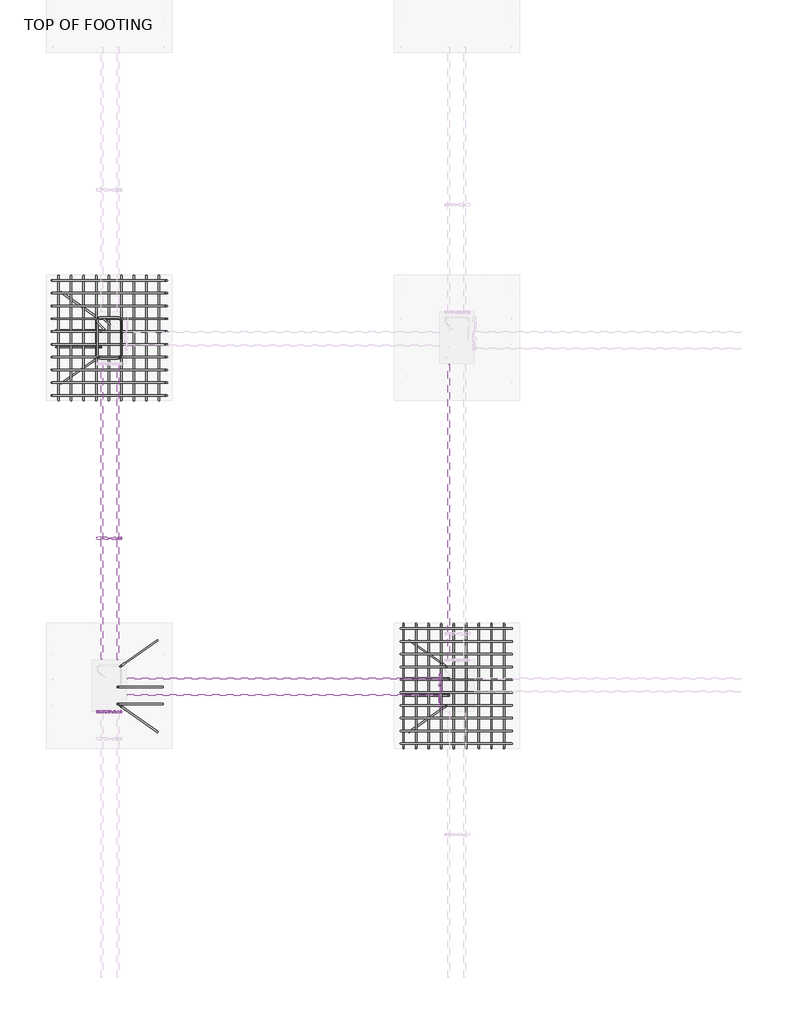
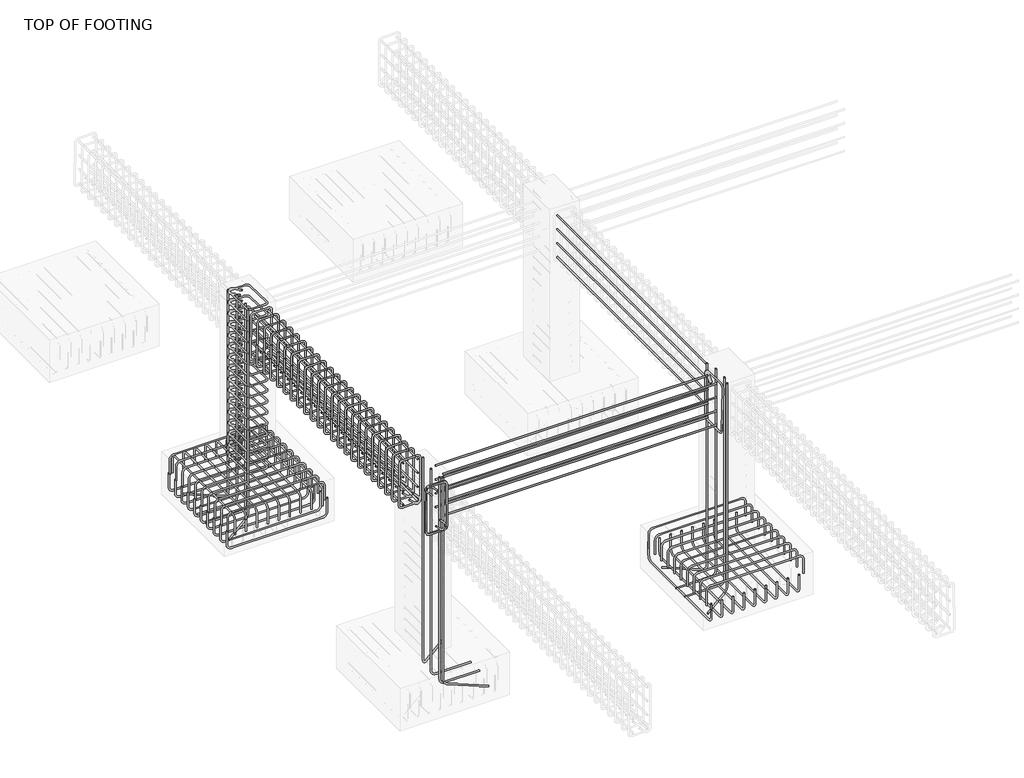
# One storey, part 6 of 18: 24 reinforcing bars.
"""IFC4 building model written with IfcOpenShell, lengths in millimetres."""

from ifc_helpers import new_model, si_unit, point, frame, origin, place, context, project, spatial, polyline, circle_curve, trimmed, segment, composite_curve, source, transform, mapped, element, save
from ifc_brep_helpers import swept_disk

model = new_model("IFC4")

# Units and contexts
model_context = context("Model", 3, world=origin())
ifc_project = project(units=[si_unit("LENGTHUNIT", "METRE", prefix="MILLI")], contexts=[model_context])

# Site, building, storey
site = spatial("IfcSite", under=ifc_project)
building = spatial("IfcBuilding", under=site)
storey = spatial("IfcBuildingStorey", under=building, Name="TOP OF FOOTING", Elevation=-1828.8)

# Reinforcing bars
placement = place(None, origin())
reinforcing_bar_shape = source(origin(), model_context, "Body", "SolidModel", [
    swept_disk(composite_curve([segment(polyline([(-11115.9859643, 12622.8477614, -40.0), (-11115.9859643, 12622.8477614, -2185.2530621)]), True, "CONTINUOUS"), segment(trimmed(circle_curve(frame((-11162.3359643, 12622.8477614, -2185.2530621), z_axis=(0.0, 1.0, 0.0), x_axis=(46.350000000000364, 0.0, 0.0)), 46.35), [point((-11115.9859643, 12622.8477614, -2185.2530621))], [point((-11162.3359643, 12622.8477614, -2231.6030621))], True, "CARTESIAN"), True, "CONTINUOUS"), segment(polyline([(-11162.3359643, 12622.8477614, -2231.6030621), (-11513.5126143, 12622.8477614, -2231.6030621)]), True, "CONTINUOUS")], self_intersect=False), 6.35),
])
element("IfcReinforcingBar", 1, at=placement, inside=storey, context=model_context, shape_type="MappedRepresentation", body=[
    mapped(reinforcing_bar_shape, transform((0.0, 0.0, 0.0), x_axis=(1.0, 0.0, 0.0), y_axis=(0.0, 1.0, 0.0), z_axis=(0.0, 0.0, 1.0))),
    mapped(reinforcing_bar_shape, transform((0.0, 148.3194112, 0.0), x_axis=(1.0, 0.0, 0.0), y_axis=(0.0, 1.0, 0.0), z_axis=(0.0, 0.0, 1.0))),
])
element("IfcReinforcingBar", 2, at=placement, inside=storey, context=model_context, shape_type="SolidModel", body=[
    swept_disk(composite_curve([segment(polyline([(-11140.9859643, 12878.3098681, -40.0), (-11140.9859643, 12878.3098681, -2185.2530621)]), True, "CONTINUOUS"), segment(trimmed(circle_curve(frame((-11178.9536616, 12904.895136, -2185.2530621), z_axis=(0.5735764363510552, 0.8191520442889856, 0.0), x_axis=(37.96769730000051, -26.585267899999963, 0.0)), 46.35), [point((-11140.9859643, 12878.3098681, -2185.2530621))], [point((-11178.9536616, 12904.895136, -2231.6030621))], True, "CARTESIAN"), True, "CONTINUOUS"), segment(polyline([(-11178.9536616, 12904.895136, -2231.6030621), (-11466.6207323, 13106.3217874, -2231.6030621)]), True, "CONTINUOUS")], self_intersect=False), 6.35),
])
reinforcing_bar_2_shape = source(origin(), model_context, "Body", "SolidModel", [
    swept_disk(composite_curve([segment(polyline([(-11036.6954038, 12818.3841028, -1782.45), (-11092.4389667, 12874.1276657, -1782.45)]), True, "CONTINUOUS"), segment(trimmed(circle_curve(frame((-11114.6067643, 12851.9598681, -1782.45), z_axis=(0.0, 0.0, 1.0), x_axis=(22.167797600000995, 22.167797599999176, 0.0)), 31.35), [point((-11092.4389667, 12874.1276657, -1782.45))], [point((-11145.9567643, 12851.9598681, -1782.45))], True, "CARTESIAN"), True, "CONTINUOUS"), segment(polyline([(-11145.9567643, 12851.9598681, -1782.45), (-11145.9567643, 12557.3598681, -1782.45)]), True, "CONTINUOUS"), segment(trimmed(circle_curve(frame((-11114.6067643, 12557.3598681, -1782.45), z_axis=(0.0, 0.0, 1.0), x_axis=(-31.349999999998545, 0.0, 0.0)), 31.35), [point((-11145.9567643, 12557.3598681, -1782.45))], [point((-11114.6067643, 12526.0098681, -1782.45))], True, "CARTESIAN"), True, "CONTINUOUS"), segment(polyline([(-11114.6067643, 12526.0098681, -1782.45), (-10970.0067643, 12526.0098681, -1782.45)]), True, "CONTINUOUS"), segment(trimmed(circle_curve(frame((-10970.0067643, 12557.3400831, -1783.5636125), z_axis=(0.0, 0.03552192833448158, 0.9993688971583016), x_axis=(0.0, -31.330214999999953, 1.1136125000000447)), 31.35), [point((-10970.0067643, 12526.0098681, -1782.45))], [point((-10938.6567643, 12557.3400831, -1783.5636125))], True, "CARTESIAN"), True, "CONTINUOUS"), segment(polyline([(-10938.6567643, 12557.3400831, -1783.5636125), (-10938.6567643, 12851.9796532, -1794.0363875)]), True, "CONTINUOUS"), segment(trimmed(circle_curve(frame((-10970.0067643, 12851.9796532, -1794.0363875), z_axis=(0.0, 0.03552192833448158, 0.9993688971583016), x_axis=(31.350000000000364, 0.0, 0.0)), 31.35), [point((-10938.6567643, 12851.9796532, -1794.0363875))], [point((-10970.0067643, 12883.3098681, -1795.15))], True, "CARTESIAN"), True, "CONTINUOUS"), segment(polyline([(-10970.0067643, 12883.3098681, -1795.15), (-11114.6067643, 12883.3098681, -1795.15)]), True, "CONTINUOUS"), segment(trimmed(circle_curve(frame((-11114.6067643, 12851.9598681, -1795.15), z_axis=(0.0, 0.0, 1.0), x_axis=(0.0, 31.349999999998545, 0.0)), 31.35), [point((-11114.6067643, 12883.3098681, -1795.15))], [point((-11136.7745619, 12829.7920705, -1795.15))], True, "CARTESIAN"), True, "CONTINUOUS"), segment(polyline([(-11136.7745619, 12829.7920705, -1795.15), (-11081.030999, 12774.0485076, -1795.15)]), True, "CONTINUOUS")], self_intersect=False), 6.35),
])
element("IfcReinforcingBar", 3, at=placement, inside=storey, context=model_context, shape_type="MappedRepresentation", body=[
    mapped(reinforcing_bar_2_shape, transform((0.0, 0.0, 0.0), x_axis=(1.0, 0.0, 0.0), y_axis=(0.0, 1.0, 0.0), z_axis=(0.0, 0.0, 1.0))),
    mapped(reinforcing_bar_2_shape, transform((0.0, 0.0, 116.0092918), x_axis=(1.0, 0.0, 0.0), y_axis=(0.0, 1.0, 0.0), z_axis=(0.0, 0.0, 1.0))),
    mapped(reinforcing_bar_2_shape, transform((0.0, 0.0, 232.0185836), x_axis=(1.0, 0.0, 0.0), y_axis=(0.0, 1.0, 0.0), z_axis=(0.0, 0.0, 1.0))),
    mapped(reinforcing_bar_2_shape, transform((0.0, 0.0, 348.0278755), x_axis=(1.0, 0.0, 0.0), y_axis=(0.0, 1.0, 0.0), z_axis=(0.0, 0.0, 1.0))),
    mapped(reinforcing_bar_2_shape, transform((0.0, 0.0, 464.0371673), x_axis=(1.0, 0.0, 0.0), y_axis=(0.0, 1.0, 0.0), z_axis=(0.0, 0.0, 1.0))),
    mapped(reinforcing_bar_2_shape, transform((0.0, 0.0, 580.0464591), x_axis=(1.0, 0.0, 0.0), y_axis=(0.0, 1.0, 0.0), z_axis=(0.0, 0.0, 1.0))),
    mapped(reinforcing_bar_2_shape, transform((0.0, 0.0, 696.0557509), x_axis=(1.0, 0.0, 0.0), y_axis=(0.0, 1.0, 0.0), z_axis=(0.0, 0.0, 1.0))),
    mapped(reinforcing_bar_2_shape, transform((0.0, 0.0, 812.0650428), x_axis=(1.0, 0.0, 0.0), y_axis=(0.0, 1.0, 0.0), z_axis=(0.0, 0.0, 1.0))),
    mapped(reinforcing_bar_2_shape, transform((0.0, 0.0, 928.0743346), x_axis=(1.0, 0.0, 0.0), y_axis=(0.0, 1.0, 0.0), z_axis=(0.0, 0.0, 1.0))),
    mapped(reinforcing_bar_2_shape, transform((0.0, 0.0, 1044.0836264), x_axis=(1.0, 0.0, 0.0), y_axis=(0.0, 1.0, 0.0), z_axis=(0.0, 0.0, 1.0))),
    mapped(reinforcing_bar_2_shape, transform((0.0, 0.0, 1160.0929182), x_axis=(1.0, 0.0, 0.0), y_axis=(0.0, 1.0, 0.0), z_axis=(0.0, 0.0, 1.0))),
    mapped(reinforcing_bar_2_shape, transform((0.0, 0.0, 1276.1022101), x_axis=(1.0, 0.0, 0.0), y_axis=(0.0, 1.0, 0.0), z_axis=(0.0, 0.0, 1.0))),
    mapped(reinforcing_bar_2_shape, transform((0.0, 0.0, 1392.1115019), x_axis=(1.0, 0.0, 0.0), y_axis=(0.0, 1.0, 0.0), z_axis=(0.0, 0.0, 1.0))),
    mapped(reinforcing_bar_2_shape, transform((0.0, 0.0, 1508.1207937), x_axis=(1.0, 0.0, 0.0), y_axis=(0.0, 1.0, 0.0), z_axis=(0.0, 0.0, 1.0))),
    mapped(reinforcing_bar_2_shape, transform((0.0, 0.0, 1624.1300855), x_axis=(1.0, 0.0, 0.0), y_axis=(0.0, 1.0, 0.0), z_axis=(0.0, 0.0, 1.0))),
    mapped(reinforcing_bar_2_shape, transform((0.0, 0.0, 1740.1393774), x_axis=(1.0, 0.0, 0.0), y_axis=(0.0, 1.0, 0.0), z_axis=(0.0, 0.0, 1.0))),
])
element("IfcReinforcingBar", 4, at=placement, inside=storey, context=model_context, shape_type="SolidModel", body=[
    swept_disk(composite_curve([segment(polyline([(-11140.9859643, 12531.0098681, -40.0), (-11140.9859643, 12531.0098681, -2185.2530621)]), True, "CONTINUOUS"), segment(trimmed(circle_curve(frame((-11178.9536616, 12504.4246003, -2185.2530621), z_axis=(-0.5735764363510106, 0.8191520442890168, 0.0), x_axis=(37.96769730000051, 26.5852677999992, 0.0)), 46.35), [point((-11140.9859643, 12531.0098681, -2185.2530621))], [point((-11178.9536616, 12504.4246003, -2231.6030621))], True, "CARTESIAN"), True, "CONTINUOUS"), segment(polyline([(-11178.9536616, 12504.4246003, -2231.6030621), (-11466.6207323, 12302.9979489, -2231.6030621)]), True, "CONTINUOUS")], self_intersect=False), 6.35),
])
element("IfcReinforcingBar", 5, at=placement, inside=storey, context=model_context, shape_type="SolidModel", body=[
    swept_disk(composite_curve([segment(polyline([(-10943.6275643, 9830.3098681, -40.0), (-10943.6275643, 9830.3098681, -2185.2530621)]), True, "CONTINUOUS"), segment(trimmed(circle_curve(frame((-10905.6598671, 9856.895136, -2185.2530621), z_axis=(0.5735764363510552, -0.8191520442889855, 0.0), x_axis=(-37.96769720000157, -26.585267899999963, 0.0)), 46.35), [point((-10943.6275643, 9830.3098681, -2185.2530621))], [point((-10905.6598671, 9856.895136, -2231.6030621))], True, "CARTESIAN"), True, "CONTINUOUS"), segment(polyline([(-10905.6598671, 9856.895136, -2231.6030621), (-10617.9927964, 10058.3217874, -2231.6030621)]), True, "CONTINUOUS")], self_intersect=False), 6.35),
])
element("IfcReinforcingBar", 6, at=placement, inside=storey, context=model_context, shape_type="SolidModel", body=[
    swept_disk(composite_curve([segment(polyline([(-10943.6275643, 9483.0098681, -40.0), (-10943.6275643, 9483.0098681, -2185.2530621)]), True, "CONTINUOUS"), segment(trimmed(circle_curve(frame((-10905.6598671, 9456.4246003, -2185.2530621), z_axis=(-0.5735764363510997, -0.8191520442889544, 0.0), x_axis=(-37.96769720000157, 26.5852677999992, 0.0)), 46.35), [point((-10943.6275643, 9483.0098681, -2185.2530621))], [point((-10905.6598671, 9456.4246003, -2231.6030621))], True, "CARTESIAN"), True, "CONTINUOUS"), segment(polyline([(-10905.6598671, 9456.4246003, -2231.6030621), (-10617.9927964, 9254.9979489, -2231.6030621)]), True, "CONTINUOUS")], self_intersect=False), 6.35),
])
reinforcing_bar_3_shape = source(origin(), model_context, "Body", "SolidModel", [
    swept_disk(composite_curve([segment(polyline([(-10968.6275643, 9499.8477614, -40.0), (-10968.6275643, 9499.8477614, -2185.2530621)]), True, "CONTINUOUS"), segment(trimmed(circle_curve(frame((-10922.2775643, 9499.8477614, -2185.2530621), z_axis=(0.0, -1.0, 0.0), x_axis=(-46.350000000000364, 0.0, 0.0)), 46.35), [point((-10968.6275643, 9499.8477614, -2185.2530621))], [point((-10922.2775643, 9499.8477614, -2231.6030621))], True, "CARTESIAN"), True, "CONTINUOUS"), segment(polyline([(-10922.2775643, 9499.8477614, -2231.6030621), (-10571.1009144, 9499.8477614, -2231.6030621)]), True, "CONTINUOUS")], self_intersect=False), 6.35),
])
element("IfcReinforcingBar", 7, at=placement, inside=storey, context=model_context, shape_type="MappedRepresentation", body=[
    mapped(reinforcing_bar_3_shape, transform((0.0, 0.0, 0.0), x_axis=(1.0, 0.0, 0.0), y_axis=(0.0, 1.0, 0.0), z_axis=(0.0, 0.0, 1.0))),
    mapped(reinforcing_bar_3_shape, transform((0.0, 148.3194112, 0.0), x_axis=(1.0, 0.0, 0.0), y_axis=(0.0, 1.0, 0.0), z_axis=(0.0, 0.0, 1.0))),
])
reinforcing_bar_4_shape = source(origin(), model_context, "Body", "SolidModel", [
    swept_disk(composite_curve([segment(polyline([(-8067.9859643, 9574.8477614, -40.0), (-8067.9859643, 9574.8477614, -2185.2530621)]), True, "CONTINUOUS"), segment(trimmed(circle_curve(frame((-8114.3359643, 9574.8477614, -2185.2530621), z_axis=(0.0, 1.0, 0.0), x_axis=(46.350000000000364, 0.0, 0.0)), 46.35), [point((-8067.9859643, 9574.8477614, -2185.2530621))], [point((-8114.3359643, 9574.8477614, -2231.6030621))], True, "CARTESIAN"), True, "CONTINUOUS"), segment(polyline([(-8114.3359643, 9574.8477614, -2231.6030621), (-8465.5126143, 9574.8477614, -2231.6030621)]), True, "CONTINUOUS")], self_intersect=False), 6.35),
])
element("IfcReinforcingBar", 8, at=placement, inside=storey, context=model_context, shape_type="MappedRepresentation", body=[
    mapped(reinforcing_bar_4_shape, transform((0.0, 0.0, 0.0), x_axis=(1.0, 0.0, 0.0), y_axis=(0.0, 1.0, 0.0), z_axis=(0.0, 0.0, 1.0))),
    mapped(reinforcing_bar_4_shape, transform((0.0, 148.3194112, 0.0), x_axis=(1.0, 0.0, 0.0), y_axis=(0.0, 1.0, 0.0), z_axis=(0.0, 0.0, 1.0))),
])
element("IfcReinforcingBar", 9, at=placement, inside=storey, context=model_context, shape_type="SolidModel", body=[
    swept_disk(composite_curve([segment(polyline([(-8092.9859643, 9830.3098681, -40.0), (-8092.9859643, 9830.3098681, -2185.2530621)]), True, "CONTINUOUS"), segment(trimmed(circle_curve(frame((-8130.9536616, 9856.895136, -2185.2530621), z_axis=(0.5735764363510552, 0.8191520442889855, 0.0), x_axis=(37.9676972999996, -26.585267899999963, 0.0)), 46.35), [point((-8092.9859643, 9830.3098681, -2185.2530621))], [point((-8130.9536616, 9856.895136, -2231.6030621))], True, "CARTESIAN"), True, "CONTINUOUS"), segment(polyline([(-8130.9536616, 9856.895136, -2231.6030621), (-8418.6207323, 10058.3217874, -2231.6030621)]), True, "CONTINUOUS")], self_intersect=False), 6.35),
])
element("IfcReinforcingBar", 10, at=placement, inside=storey, context=model_context, shape_type="SolidModel", body=[
    swept_disk(composite_curve([segment(polyline([(-8092.9859643, 9483.0098681, -40.0), (-8092.9859643, 9483.0098681, -2185.2530621)]), True, "CONTINUOUS"), segment(trimmed(circle_curve(frame((-8130.9536616, 9456.4246003, -2185.2530621), z_axis=(-0.5735764363510105, 0.8191520442890168, 0.0), x_axis=(37.9676972999996, 26.5852677999992, 0.0)), 46.35), [point((-8092.9859643, 9483.0098681, -2185.2530621))], [point((-8130.9536616, 9456.4246003, -2231.6030621))], True, "CARTESIAN"), True, "CONTINUOUS"), segment(polyline([(-8130.9536616, 9456.4246003, -2231.6030621), (-8418.6207323, 9254.9979489, -2231.6030621)]), True, "CONTINUOUS")], self_intersect=False), 6.35),
])
reinforcing_bar_5_shape = source(origin(), model_context, "Body", "SolidModel", [
    swept_disk(composite_curve([segment(polyline([(-8488.4399078, 10160.3098681, -2056.7800629), (-8488.4399078, 10160.3098681, -1909.4800629)]), True, "CONTINUOUS"), segment(trimmed(circle_curve(frame((-8442.0899078, 10160.3098681, -1909.4800629), z_axis=(0.0, 1.0, 0.0), x_axis=(-46.350000000000364, 0.0, 0.0)), 46.35), [point((-8488.4399078, 10160.3098681, -1909.4800629))], [point((-8442.0899078, 10160.3098681, -1863.1300629))], True, "CARTESIAN"), True, "CONTINUOUS"), segment(polyline([(-8442.0899078, 10160.3098681, -1863.1300629), (-7562.3320898, 10160.3098681, -1863.1300629)]), True, "CONTINUOUS"), segment(trimmed(circle_curve(frame((-7562.3320898, 10160.3098681, -1909.4800629), z_axis=(0.0, 1.0, 0.0), x_axis=(0.0, 0.0, 46.34999999999991)), 46.35), [point((-7562.3320898, 10160.3098681, -1863.1300629))], [point((-7515.9820898, 10160.3098681, -1909.4800629))], True, "CARTESIAN"), True, "CONTINUOUS"), segment(polyline([(-7515.9820898, 10160.3098681, -1909.4800629), (-7515.9820898, 10160.3098681, -2056.7800629)]), True, "CONTINUOUS")], self_intersect=False), 6.35),
])
element("IfcReinforcingBar", 11, at=placement, inside=storey, context=model_context, shape_type="MappedRepresentation", body=[
    mapped(reinforcing_bar_5_shape, transform((0.0, 0.0, 0.0), x_axis=(1.0, 0.0, 0.0), y_axis=(0.0, 1.0, 0.0), z_axis=(0.0, 0.0, 1.0))),
    mapped(reinforcing_bar_5_shape, transform((0.0, -111.9222222, 0.0), x_axis=(1.0, 0.0, 0.0), y_axis=(0.0, 1.0, 0.0), z_axis=(0.0, 0.0, 1.0))),
    mapped(reinforcing_bar_5_shape, transform((0.0, -223.8444444, 0.0), x_axis=(1.0, 0.0, 0.0), y_axis=(0.0, 1.0, 0.0), z_axis=(0.0, 0.0, 1.0))),
    mapped(reinforcing_bar_5_shape, transform((0.0, -335.7666667, 0.0), x_axis=(1.0, 0.0, 0.0), y_axis=(0.0, 1.0, 0.0), z_axis=(0.0, 0.0, 1.0))),
    mapped(reinforcing_bar_5_shape, transform((0.0, -447.6888889, 0.0), x_axis=(1.0, 0.0, 0.0), y_axis=(0.0, 1.0, 0.0), z_axis=(0.0, 0.0, 1.0))),
    mapped(reinforcing_bar_5_shape, transform((0.0, -559.6111111, 0.0), x_axis=(1.0, 0.0, 0.0), y_axis=(0.0, 1.0, 0.0), z_axis=(0.0, 0.0, 1.0))),
    mapped(reinforcing_bar_5_shape, transform((0.0, -671.5333333, 0.0), x_axis=(1.0, 0.0, 0.0), y_axis=(0.0, 1.0, 0.0), z_axis=(0.0, 0.0, 1.0))),
    mapped(reinforcing_bar_5_shape, transform((0.0, -783.4555556, 0.0), x_axis=(1.0, 0.0, 0.0), y_axis=(0.0, 1.0, 0.0), z_axis=(0.0, 0.0, 1.0))),
    mapped(reinforcing_bar_5_shape, transform((0.0, -895.3777778, 0.0), x_axis=(1.0, 0.0, 0.0), y_axis=(0.0, 1.0, 0.0), z_axis=(0.0, 0.0, 1.0))),
    mapped(reinforcing_bar_5_shape, transform((0.0, -1007.3, 0.0), x_axis=(1.0, 0.0, 0.0), y_axis=(0.0, 1.0, 0.0), z_axis=(0.0, 0.0, 1.0))),
])
reinforcing_bar_6_shape = source(origin(), model_context, "Body", "SolidModel", [
    swept_disk(composite_curve([segment(polyline([(-8465.5126143, 10200.3098681, -2025.2530621), (-8465.5126143, 10200.3098681, -2172.5530621)]), True, "CONTINUOUS"), segment(trimmed(circle_curve(frame((-8465.5126143, 10153.9598681, -2172.5530621), z_axis=(-1.0, 0.0, 0.0), x_axis=(0.0, 46.349999999998545, 0.0)), 46.35), [point((-8465.5126143, 10200.3098681, -2172.5530621))], [point((-8465.5126143, 10153.9598681, -2218.9030621))], True, "CARTESIAN"), True, "CONTINUOUS"), segment(polyline([(-8465.5126143, 10153.9598681, -2218.9030621), (-8465.5126143, 9159.3598681, -2218.9030621)]), True, "CONTINUOUS"), segment(trimmed(circle_curve(frame((-8465.5126143, 9159.3598681, -2172.5530621), z_axis=(-1.0, 0.0, 0.0), x_axis=(0.0, 0.0, -46.350000000000364)), 46.35), [point((-8465.5126143, 9159.3598681, -2218.9030621))], [point((-8465.5126143, 9113.0098681, -2172.5530621))], True, "CARTESIAN"), True, "CONTINUOUS"), segment(polyline([(-8465.5126143, 9113.0098681, -2172.5530621), (-8465.5126143, 9113.0098681, -2025.2530621)]), True, "CONTINUOUS")], self_intersect=False), 6.35),
])
element("IfcReinforcingBar", 12, at=placement, inside=storey, context=model_context, shape_type="MappedRepresentation", body=[
    mapped(reinforcing_bar_6_shape, transform((0.0, 0.0, 0.0), x_axis=(1.0, 0.0, 0.0), y_axis=(0.0, 1.0, 0.0), z_axis=(0.0, 0.0, 1.0))),
    mapped(reinforcing_bar_6_shape, transform((109.9890349, 0.0, 0.0), x_axis=(1.0, 0.0, 0.0), y_axis=(0.0, 1.0, 0.0), z_axis=(0.0, 0.0, 1.0))),
    mapped(reinforcing_bar_6_shape, transform((219.9780699, 0.0, 0.0), x_axis=(1.0, 0.0, 0.0), y_axis=(0.0, 1.0, 0.0), z_axis=(0.0, 0.0, 1.0))),
    mapped(reinforcing_bar_6_shape, transform((329.9671048, 0.0, 0.0), x_axis=(1.0, 0.0, 0.0), y_axis=(0.0, 1.0, 0.0), z_axis=(0.0, 0.0, 1.0))),
    mapped(reinforcing_bar_6_shape, transform((439.9561397, 0.0, 0.0), x_axis=(1.0, 0.0, 0.0), y_axis=(0.0, 1.0, 0.0), z_axis=(0.0, 0.0, 1.0))),
    mapped(reinforcing_bar_6_shape, transform((549.9451746, 0.0, 0.0), x_axis=(1.0, 0.0, 0.0), y_axis=(0.0, 1.0, 0.0), z_axis=(0.0, 0.0, 1.0))),
    mapped(reinforcing_bar_6_shape, transform((659.9342096, 0.0, 0.0), x_axis=(1.0, 0.0, 0.0), y_axis=(0.0, 1.0, 0.0), z_axis=(0.0, 0.0, 1.0))),
    mapped(reinforcing_bar_6_shape, transform((769.9232445, 0.0, 0.0), x_axis=(1.0, 0.0, 0.0), y_axis=(0.0, 1.0, 0.0), z_axis=(0.0, 0.0, 1.0))),
    mapped(reinforcing_bar_6_shape, transform((879.9122794, 0.0, 0.0), x_axis=(1.0, 0.0, 0.0), y_axis=(0.0, 1.0, 0.0), z_axis=(0.0, 0.0, 1.0))),
])
reinforcing_bar_7_shape = source(origin(), model_context, "Body", "SolidModel", [
    swept_disk(composite_curve([segment(polyline([(-10538.6567643, 13208.3098681, -2046.8654906), (-10538.6567643, 13208.3098681, -2194.1654906)]), True, "CONTINUOUS"), segment(trimmed(circle_curve(frame((-10585.0067643, 13208.3098681, -2194.1654906), z_axis=(0.0, 1.0, 0.0), x_axis=(46.350000000000364, 0.0, 0.0)), 46.35), [point((-10538.6567643, 13208.3098681, -2194.1654906))], [point((-10585.0067643, 13208.3098681, -2240.5154906))], True, "CARTESIAN"), True, "CONTINUOUS"), segment(polyline([(-10585.0067643, 13208.3098681, -2240.5154906), (-11499.6067643, 13208.3098681, -2240.5154906)]), True, "CONTINUOUS"), segment(trimmed(circle_curve(frame((-11499.6067643, 13208.3098681, -2194.1654906), z_axis=(0.0, 1.0, 0.0), x_axis=(0.0, 0.0, -46.34999999999991)), 46.35), [point((-11499.6067643, 13208.3098681, -2240.5154906))], [point((-11545.9567643, 13208.3098681, -2194.1654906))], True, "CARTESIAN"), True, "CONTINUOUS"), segment(polyline([(-11545.9567643, 13208.3098681, -2194.1654906), (-11545.9567643, 13208.3098681, -2046.8654906)]), True, "CONTINUOUS")], self_intersect=False), 6.35),
])
element("IfcReinforcingBar", 13, at=placement, inside=storey, context=model_context, shape_type="MappedRepresentation", body=[
    mapped(reinforcing_bar_7_shape, transform((0.0, 0.0, 0.0), x_axis=(1.0, 0.0, 0.0), y_axis=(0.0, 1.0, 0.0), z_axis=(0.0, 0.0, 1.0))),
    mapped(reinforcing_bar_7_shape, transform((0.0, -111.9222222, 0.0), x_axis=(1.0, 0.0, 0.0), y_axis=(0.0, 1.0, 0.0), z_axis=(0.0, 0.0, 1.0))),
    mapped(reinforcing_bar_7_shape, transform((0.0, -223.8444444, 0.0), x_axis=(1.0, 0.0, 0.0), y_axis=(0.0, 1.0, 0.0), z_axis=(0.0, 0.0, 1.0))),
    mapped(reinforcing_bar_7_shape, transform((0.0, -335.7666667, 0.0), x_axis=(1.0, 0.0, 0.0), y_axis=(0.0, 1.0, 0.0), z_axis=(0.0, 0.0, 1.0))),
    mapped(reinforcing_bar_7_shape, transform((0.0, -447.6888889, 0.0), x_axis=(1.0, 0.0, 0.0), y_axis=(0.0, 1.0, 0.0), z_axis=(0.0, 0.0, 1.0))),
    mapped(reinforcing_bar_7_shape, transform((0.0, -559.6111111, 0.0), x_axis=(1.0, 0.0, 0.0), y_axis=(0.0, 1.0, 0.0), z_axis=(0.0, 0.0, 1.0))),
    mapped(reinforcing_bar_7_shape, transform((0.0, -671.5333333, 0.0), x_axis=(1.0, 0.0, 0.0), y_axis=(0.0, 1.0, 0.0), z_axis=(0.0, 0.0, 1.0))),
    mapped(reinforcing_bar_7_shape, transform((0.0, -783.4555556, 0.0), x_axis=(1.0, 0.0, 0.0), y_axis=(0.0, 1.0, 0.0), z_axis=(0.0, 0.0, 1.0))),
    mapped(reinforcing_bar_7_shape, transform((0.0, -895.3777778, 0.0), x_axis=(1.0, 0.0, 0.0), y_axis=(0.0, 1.0, 0.0), z_axis=(0.0, 0.0, 1.0))),
    mapped(reinforcing_bar_7_shape, transform((0.0, -1007.3, 0.0), x_axis=(1.0, 0.0, 0.0), y_axis=(0.0, 1.0, 0.0), z_axis=(0.0, 0.0, 1.0))),
])
reinforcing_bar_8_shape = source(origin(), model_context, "Body", "SolidModel", [
    swept_disk(composite_curve([segment(polyline([(-11536.4399078, 13208.3098681, -2056.7800629), (-11536.4399078, 13208.3098681, -1909.4800629)]), True, "CONTINUOUS"), segment(trimmed(circle_curve(frame((-11490.0899078, 13208.3098681, -1909.4800629), z_axis=(0.0, 1.0, 0.0), x_axis=(-46.350000000000364, 0.0, 0.0)), 46.35), [point((-11536.4399078, 13208.3098681, -1909.4800629))], [point((-11490.0899078, 13208.3098681, -1863.1300629))], True, "CARTESIAN"), True, "CONTINUOUS"), segment(polyline([(-11490.0899078, 13208.3098681, -1863.1300629), (-10610.3320898, 13208.3098681, -1863.1300629)]), True, "CONTINUOUS"), segment(trimmed(circle_curve(frame((-10610.3320898, 13208.3098681, -1909.4800629), z_axis=(0.0, 1.0, 0.0), x_axis=(0.0, 0.0, 46.34999999999991)), 46.35), [point((-10610.3320898, 13208.3098681, -1863.1300629))], [point((-10563.9820898, 13208.3098681, -1909.4800629))], True, "CARTESIAN"), True, "CONTINUOUS"), segment(polyline([(-10563.9820898, 13208.3098681, -1909.4800629), (-10563.9820898, 13208.3098681, -2056.7800629)]), True, "CONTINUOUS")], self_intersect=False), 6.35),
])
element("IfcReinforcingBar", 14, at=placement, inside=storey, context=model_context, shape_type="MappedRepresentation", body=[
    mapped(reinforcing_bar_8_shape, transform((0.0, 0.0, 0.0), x_axis=(1.0, 0.0, 0.0), y_axis=(0.0, 1.0, 0.0), z_axis=(0.0, 0.0, 1.0))),
    mapped(reinforcing_bar_8_shape, transform((0.0, -111.9222222, 0.0), x_axis=(1.0, 0.0, 0.0), y_axis=(0.0, 1.0, 0.0), z_axis=(0.0, 0.0, 1.0))),
    mapped(reinforcing_bar_8_shape, transform((0.0, -223.8444444, 0.0), x_axis=(1.0, 0.0, 0.0), y_axis=(0.0, 1.0, 0.0), z_axis=(0.0, 0.0, 1.0))),
    mapped(reinforcing_bar_8_shape, transform((0.0, -335.7666667, 0.0), x_axis=(1.0, 0.0, 0.0), y_axis=(0.0, 1.0, 0.0), z_axis=(0.0, 0.0, 1.0))),
    mapped(reinforcing_bar_8_shape, transform((0.0, -447.6888889, 0.0), x_axis=(1.0, 0.0, 0.0), y_axis=(0.0, 1.0, 0.0), z_axis=(0.0, 0.0, 1.0))),
    mapped(reinforcing_bar_8_shape, transform((0.0, -559.6111111, 0.0), x_axis=(1.0, 0.0, 0.0), y_axis=(0.0, 1.0, 0.0), z_axis=(0.0, 0.0, 1.0))),
    mapped(reinforcing_bar_8_shape, transform((0.0, -671.5333333, 0.0), x_axis=(1.0, 0.0, 0.0), y_axis=(0.0, 1.0, 0.0), z_axis=(0.0, 0.0, 1.0))),
    mapped(reinforcing_bar_8_shape, transform((0.0, -783.4555556, 0.0), x_axis=(1.0, 0.0, 0.0), y_axis=(0.0, 1.0, 0.0), z_axis=(0.0, 0.0, 1.0))),
    mapped(reinforcing_bar_8_shape, transform((0.0, -895.3777778, 0.0), x_axis=(1.0, 0.0, 0.0), y_axis=(0.0, 1.0, 0.0), z_axis=(0.0, 0.0, 1.0))),
    mapped(reinforcing_bar_8_shape, transform((0.0, -1007.3, 0.0), x_axis=(1.0, 0.0, 0.0), y_axis=(0.0, 1.0, 0.0), z_axis=(0.0, 0.0, 1.0))),
])
reinforcing_bar_9_shape = source(origin(), model_context, "Body", "SolidModel", [
    swept_disk(composite_curve([segment(polyline([(-10607.1065918, 13248.3098681, -2080.1793981), (-10607.1065918, 13248.3098681, -1932.8793981)]), True, "CONTINUOUS"), segment(trimmed(circle_curve(frame((-10607.1065918, 13201.9598681, -1932.8793981), z_axis=(1.0, 0.0, 0.0), x_axis=(0.0, 46.349999999998545, 0.0)), 46.35), [point((-10607.1065918, 13248.3098681, -1932.8793981))], [point((-10607.1065918, 13201.9598681, -1886.5293981))], True, "CARTESIAN"), True, "CONTINUOUS"), segment(polyline([(-10607.1065918, 13201.9598681, -1886.5293981), (-10607.1065918, 12207.3598681, -1886.5293981)]), True, "CONTINUOUS"), segment(trimmed(circle_curve(frame((-10607.1065918, 12207.3598681, -1932.8793981), z_axis=(1.0, 0.0, 0.0), x_axis=(0.0, 0.0, 46.34999999999991)), 46.35), [point((-10607.1065918, 12207.3598681, -1886.5293981))], [point((-10607.1065918, 12161.0098681, -1932.8793981))], True, "CARTESIAN"), True, "CONTINUOUS"), segment(polyline([(-10607.1065918, 12161.0098681, -1932.8793981), (-10607.1065918, 12161.0098681, -2080.1793981)]), True, "CONTINUOUS")], self_intersect=False), 6.35),
])
element("IfcReinforcingBar", 15, at=placement, inside=storey, context=model_context, shape_type="MappedRepresentation", body=[
    mapped(reinforcing_bar_9_shape, transform((0.0, 0.0, 0.0), x_axis=(1.0, 0.0, 0.0), y_axis=(0.0, 1.0, 0.0), z_axis=(0.0, 0.0, 1.0))),
    mapped(reinforcing_bar_9_shape, transform((-109.9785589, 0.0, 0.0), x_axis=(1.0, 0.0, 0.0), y_axis=(0.0, 1.0, 0.0), z_axis=(0.0, 0.0, 1.0))),
    mapped(reinforcing_bar_9_shape, transform((-219.9571177, 0.0, 0.0), x_axis=(1.0, 0.0, 0.0), y_axis=(0.0, 1.0, 0.0), z_axis=(0.0, 0.0, 1.0))),
    mapped(reinforcing_bar_9_shape, transform((-329.9356766, 0.0, 0.0), x_axis=(1.0, 0.0, 0.0), y_axis=(0.0, 1.0, 0.0), z_axis=(0.0, 0.0, 1.0))),
    mapped(reinforcing_bar_9_shape, transform((-439.9142355, 0.0, 0.0), x_axis=(1.0, 0.0, 0.0), y_axis=(0.0, 1.0, 0.0), z_axis=(0.0, 0.0, 1.0))),
    mapped(reinforcing_bar_9_shape, transform((-549.8927943, 0.0, 0.0), x_axis=(1.0, 0.0, 0.0), y_axis=(0.0, 1.0, 0.0), z_axis=(0.0, 0.0, 1.0))),
    mapped(reinforcing_bar_9_shape, transform((-659.8713532, 0.0, 0.0), x_axis=(1.0, 0.0, 0.0), y_axis=(0.0, 1.0, 0.0), z_axis=(0.0, 0.0, 1.0))),
    mapped(reinforcing_bar_9_shape, transform((-769.8499121, 0.0, 0.0), x_axis=(1.0, 0.0, 0.0), y_axis=(0.0, 1.0, 0.0), z_axis=(0.0, 0.0, 1.0))),
    mapped(reinforcing_bar_9_shape, transform((-879.828471, 0.0, 0.0), x_axis=(1.0, 0.0, 0.0), y_axis=(0.0, 1.0, 0.0), z_axis=(0.0, 0.0, 1.0))),
])
reinforcing_bar_10_shape = source(origin(), model_context, "Body", "SolidModel", [
    swept_disk(composite_curve([segment(polyline([(-11047.9181249, 12473.3098681, -488.7242346), (-10992.1745619, 12473.3098681, -544.4677976)]), True, "CONTINUOUS"), segment(trimmed(circle_curve(frame((-10970.0067643, 12473.3098681, -522.3), z_axis=(0.0, -1.0, 0.0), x_axis=(-22.167797599999176, 0.0, -22.167797600000085)), 31.35), [point((-10992.1745619, 12473.3098681, -544.4677976))], [point((-10938.6567643, 12473.3098681, -522.3))], True, "CARTESIAN"), True, "CONTINUOUS"), segment(polyline([(-10938.6567643, 12473.3098681, -522.3), (-10938.6567643, 12473.3098681, -77.7)]), True, "CONTINUOUS"), segment(trimmed(circle_curve(frame((-10970.0067643, 12473.3098681, -77.7), z_axis=(0.0, -1.0, 0.0), x_axis=(31.350000000000364, 0.0, 0.0)), 31.35), [point((-10938.6567643, 12473.3098681, -77.7))], [point((-10970.0067643, 12473.3098681, -46.35))], True, "CARTESIAN"), True, "CONTINUOUS"), segment(polyline([(-10970.0067643, 12473.3098681, -46.35), (-11114.6067643, 12473.3098681, -46.35)]), True, "CONTINUOUS"), segment(trimmed(circle_curve(frame((-11114.6067643, 12474.0944538, -77.6901807), z_axis=(0.0, -0.9996867842138424, -0.025026655153786322), x_axis=(0.0, -0.7845857000011165, 31.340180699999998)), 31.35), [point((-11114.6067643, 12473.3098681, -46.35))], [point((-11145.9567643, 12474.0944538, -77.6901807))], True, "CARTESIAN"), True, "CONTINUOUS"), segment(polyline([(-11145.9567643, 12474.0944538, -77.6901807), (-11145.9567643, 12485.2252825, -522.3098193)]), True, "CONTINUOUS"), segment(trimmed(circle_curve(frame((-11114.6067643, 12485.2252825, -522.3098193), z_axis=(0.0, -0.9996867842138424, -0.025026655153786322), x_axis=(-31.349999999998545, 0.0, 0.0)), 31.35), [point((-11145.9567643, 12485.2252825, -522.3098193))], [point((-11114.6067643, 12486.0098681, -553.65))], True, "CARTESIAN"), True, "CONTINUOUS"), segment(polyline([(-11114.6067643, 12486.0098681, -553.65), (-10970.0067643, 12486.0098681, -553.65)]), True, "CONTINUOUS"), segment(trimmed(circle_curve(frame((-10970.0067643, 12486.0098681, -522.3), z_axis=(0.0, -1.0, 0.0), x_axis=(0.0, 0.0, -31.350000000000023)), 31.35), [point((-10970.0067643, 12486.0098681, -553.65))], [point((-10947.8389667, 12486.0098681, -500.1322024))], True, "CARTESIAN"), True, "CONTINUOUS"), segment(polyline([(-10947.8389667, 12486.0098681, -500.1322024), (-11003.5825297, 12486.0098681, -444.3886395)]), True, "CONTINUOUS")], self_intersect=False), 6.35),
])
element("IfcReinforcingBar", 16, at=placement, inside=storey, context=model_context, shape_type="MappedRepresentation", body=[
    mapped(reinforcing_bar_10_shape, transform((0.0, 0.0, 0.0), x_axis=(1.0, 0.0, 0.0), y_axis=(0.0, 1.0, 0.0), z_axis=(0.0, 0.0, 1.0))),
    mapped(reinforcing_bar_10_shape, transform((0.0, -117.5136364, 0.0), x_axis=(1.0, 0.0, 0.0), y_axis=(0.0, 1.0, 0.0), z_axis=(0.0, 0.0, 1.0))),
    mapped(reinforcing_bar_10_shape, transform((0.0, -235.0272727, 0.0), x_axis=(1.0, 0.0, 0.0), y_axis=(0.0, 1.0, 0.0), z_axis=(0.0, 0.0, 1.0))),
    mapped(reinforcing_bar_10_shape, transform((0.0, -352.5409091, 0.0), x_axis=(1.0, 0.0, 0.0), y_axis=(0.0, 1.0, 0.0), z_axis=(0.0, 0.0, 1.0))),
    mapped(reinforcing_bar_10_shape, transform((0.0, -470.0545455, 0.0), x_axis=(1.0, 0.0, 0.0), y_axis=(0.0, 1.0, 0.0), z_axis=(0.0, 0.0, 1.0))),
    mapped(reinforcing_bar_10_shape, transform((0.0, -587.5681818, 0.0), x_axis=(1.0, 0.0, 0.0), y_axis=(0.0, 1.0, 0.0), z_axis=(0.0, 0.0, 1.0))),
    mapped(reinforcing_bar_10_shape, transform((0.0, -705.0818182, 0.0), x_axis=(1.0, 0.0, 0.0), y_axis=(0.0, 1.0, 0.0), z_axis=(0.0, 0.0, 1.0))),
    mapped(reinforcing_bar_10_shape, transform((0.0, -822.5954545, 0.0), x_axis=(1.0, 0.0, 0.0), y_axis=(0.0, 1.0, 0.0), z_axis=(0.0, 0.0, 1.0))),
    mapped(reinforcing_bar_10_shape, transform((0.0, -940.1090909, 0.0), x_axis=(1.0, 0.0, 0.0), y_axis=(0.0, 1.0, 0.0), z_axis=(0.0, 0.0, 1.0))),
    mapped(reinforcing_bar_10_shape, transform((0.0, -1057.6227273, 0.0), x_axis=(1.0, 0.0, 0.0), y_axis=(0.0, 1.0, 0.0), z_axis=(0.0, 0.0, 1.0))),
    mapped(reinforcing_bar_10_shape, transform((0.0, -1175.1363636, 0.0), x_axis=(1.0, 0.0, 0.0), y_axis=(0.0, 1.0, 0.0), z_axis=(0.0, 0.0, 1.0))),
    mapped(reinforcing_bar_10_shape, transform((0.0, -1292.65, 0.0), x_axis=(1.0, 0.0, 0.0), y_axis=(0.0, 1.0, 0.0), z_axis=(0.0, 0.0, 1.0))),
    mapped(reinforcing_bar_10_shape, transform((0.0, -1410.1636364, 0.0), x_axis=(1.0, 0.0, 0.0), y_axis=(0.0, 1.0, 0.0), z_axis=(0.0, 0.0, 1.0))),
    mapped(reinforcing_bar_10_shape, transform((0.0, -1527.6772727, 0.0), x_axis=(1.0, 0.0, 0.0), y_axis=(0.0, 1.0, 0.0), z_axis=(0.0, 0.0, 1.0))),
    mapped(reinforcing_bar_10_shape, transform((0.0, -1645.1909091, 0.0), x_axis=(1.0, 0.0, 0.0), y_axis=(0.0, 1.0, 0.0), z_axis=(0.0, 0.0, 1.0))),
    mapped(reinforcing_bar_10_shape, transform((0.0, -1762.7045455, 0.0), x_axis=(1.0, 0.0, 0.0), y_axis=(0.0, 1.0, 0.0), z_axis=(0.0, 0.0, 1.0))),
    mapped(reinforcing_bar_10_shape, transform((0.0, -1880.2181818, 0.0), x_axis=(1.0, 0.0, 0.0), y_axis=(0.0, 1.0, 0.0), z_axis=(0.0, 0.0, 1.0))),
    mapped(reinforcing_bar_10_shape, transform((0.0, -1997.7318182, 0.0), x_axis=(1.0, 0.0, 0.0), y_axis=(0.0, 1.0, 0.0), z_axis=(0.0, 0.0, 1.0))),
    mapped(reinforcing_bar_10_shape, transform((0.0, -2115.2454545, 0.0), x_axis=(1.0, 0.0, 0.0), y_axis=(0.0, 1.0, 0.0), z_axis=(0.0, 0.0, 1.0))),
    mapped(reinforcing_bar_10_shape, transform((0.0, -2232.7590909, 0.0), x_axis=(1.0, 0.0, 0.0), y_axis=(0.0, 1.0, 0.0), z_axis=(0.0, 0.0, 1.0))),
    mapped(reinforcing_bar_10_shape, transform((0.0, -2350.2727273, 0.0), x_axis=(1.0, 0.0, 0.0), y_axis=(0.0, 1.0, 0.0), z_axis=(0.0, 0.0, 1.0))),
    mapped(reinforcing_bar_10_shape, transform((0.0, -2467.7863636, 0.0), x_axis=(1.0, 0.0, 0.0), y_axis=(0.0, 1.0, 0.0), z_axis=(0.0, 0.0, 1.0))),
    mapped(reinforcing_bar_10_shape, transform((0.0, -2585.3, 0.0), x_axis=(1.0, 0.0, 0.0), y_axis=(0.0, 1.0, 0.0), z_axis=(0.0, 0.0, 1.0))),
])
reinforcing_bar_11_shape = source(origin(), model_context, "Body", "SolidModel", [
    swept_disk(composite_curve([segment(polyline([(-10966.3740978, 12479.2648964, -524.1097861), (-10966.3740978, 9885.958437, -524.1097861)]), True, "CONTINUOUS")], self_intersect=False), 6.35),
])
element("IfcReinforcingBar", 17, at=placement, inside=storey, context=model_context, shape_type="MappedRepresentation", body=[
    mapped(reinforcing_bar_11_shape, transform((0.0, 0.0, 0.0), x_axis=(1.0, 0.0, 0.0), y_axis=(0.0, 1.0, 0.0), z_axis=(0.0, 0.0, 1.0))),
    mapped(reinforcing_bar_11_shape, transform((0.0, 0.0, 147.1005596), x_axis=(1.0, 0.0, 0.0), y_axis=(0.0, 1.0, 0.0), z_axis=(0.0, 0.0, 1.0))),
    mapped(reinforcing_bar_11_shape, transform((0.0, 0.0, 294.2011193), x_axis=(1.0, 0.0, 0.0), y_axis=(0.0, 1.0, 0.0), z_axis=(0.0, 0.0, 1.0))),
    mapped(reinforcing_bar_11_shape, transform((0.0, 0.0, 441.3016789), x_axis=(1.0, 0.0, 0.0), y_axis=(0.0, 1.0, 0.0), z_axis=(0.0, 0.0, 1.0))),
])
reinforcing_bar_12_shape = source(origin(), model_context, "Body", "SolidModel", [
    swept_disk(composite_curve([segment(polyline([(-11108.2394308, 12474.6455035, -524.1097861), (-11108.2394308, 9891.9745179, -524.1097861)]), True, "CONTINUOUS")], self_intersect=False), 6.35),
])
element("IfcReinforcingBar", 18, at=placement, inside=storey, context=model_context, shape_type="MappedRepresentation", body=[
    mapped(reinforcing_bar_12_shape, transform((0.0, 0.0, 0.0), x_axis=(1.0, 0.0, 0.0), y_axis=(0.0, 1.0, 0.0), z_axis=(0.0, 0.0, 1.0))),
    mapped(reinforcing_bar_12_shape, transform((0.0, 0.0, 147.1005596), x_axis=(1.0, 0.0, 0.0), y_axis=(0.0, 1.0, 0.0), z_axis=(0.0, 0.0, 1.0))),
    mapped(reinforcing_bar_12_shape, transform((0.0, 0.0, 294.2011193), x_axis=(1.0, 0.0, 0.0), y_axis=(0.0, 1.0, 0.0), z_axis=(0.0, 0.0, 1.0))),
    mapped(reinforcing_bar_12_shape, transform((0.0, 0.0, 441.3016789), x_axis=(1.0, 0.0, 0.0), y_axis=(0.0, 1.0, 0.0), z_axis=(0.0, 0.0, 1.0))),
])
element("IfcReinforcingBar", 19, at=placement, inside=storey, context=model_context, shape_type="SolidModel", body=[
    swept_disk(composite_curve([segment(polyline([(-11036.6954038, 9425.3098681, -111.2757654), (-11092.4389667, 9425.3098681, -55.5322024)]), True, "CONTINUOUS"), segment(trimmed(circle_curve(frame((-11114.6067643, 9425.3098681, -77.7), z_axis=(0.0, -1.0, 0.0), x_axis=(22.167797600000995, 0.0, 22.1677976)), 31.35), [point((-11092.4389667, 9425.3098681, -55.5322024))], [point((-11145.9567643, 9425.3098681, -77.7))], True, "CARTESIAN"), True, "CONTINUOUS"), segment(polyline([(-11145.9567643, 9425.3098681, -77.7), (-11145.9567643, 9425.3098681, -522.3)]), True, "CONTINUOUS"), segment(trimmed(circle_curve(frame((-11114.6067643, 9425.3098681, -522.3), z_axis=(0.0, -1.0, 0.0), x_axis=(-31.349999999998545, 0.0, 0.0)), 31.35), [point((-11145.9567643, 9425.3098681, -522.3))], [point((-11114.6067643, 9425.3098681, -553.65))], True, "CARTESIAN"), True, "CONTINUOUS"), segment(polyline([(-11114.6067643, 9425.3098681, -553.65), (-10970.0067643, 9425.3098681, -553.65)]), True, "CONTINUOUS"), segment(trimmed(circle_curve(frame((-10970.0067643, 9426.0944538, -522.3098193), z_axis=(0.0, -0.9996867842138424, 0.025026655153786322), x_axis=(0.0, -0.7845857000011165, -31.34018070000002)), 31.35), [point((-10970.0067643, 9425.3098681, -553.65))], [point((-10938.6567643, 9426.0944538, -522.3098193))], True, "CARTESIAN"), True, "CONTINUOUS"), segment(polyline([(-10938.6567643, 9426.0944538, -522.3098193), (-10938.6567643, 9437.2252825, -77.6901807)]), True, "CONTINUOUS"), segment(trimmed(circle_curve(frame((-10970.0067643, 9437.2252825, -77.6901807), z_axis=(0.0, -0.9996867842138424, 0.025026655153786322), x_axis=(31.350000000000364, 0.0, 0.0)), 31.35), [point((-10938.6567643, 9437.2252825, -77.6901807))], [point((-10970.0067643, 9438.0098681, -46.35))], True, "CARTESIAN"), True, "CONTINUOUS"), segment(polyline([(-10970.0067643, 9438.0098681, -46.35), (-11114.6067643, 9438.0098681, -46.35)]), True, "CONTINUOUS"), segment(trimmed(circle_curve(frame((-11114.6067643, 9438.0098681, -77.7), z_axis=(0.0, -1.0, 0.0), x_axis=(0.0, 0.0, 31.35)), 31.35), [point((-11114.6067643, 9438.0098681, -46.35))], [point((-11136.7745619, 9438.0098681, -99.8677976))], True, "CARTESIAN"), True, "CONTINUOUS"), segment(polyline([(-11136.7745619, 9438.0098681, -99.8677976), (-11081.030999, 9438.0098681, -155.6113605)]), True, "CONTINUOUS")], self_intersect=False), 6.35),
])
element("IfcReinforcingBar", 20, at=placement, inside=storey, context=model_context, shape_type="SolidModel", body=[
    swept_disk(composite_curve([segment(polyline([(-11047.9181249, 9425.3098681, -488.7242346), (-10992.1745619, 9425.3098681, -544.4677976)]), True, "CONTINUOUS"), segment(trimmed(circle_curve(frame((-10970.0067643, 9425.3098681, -522.3), z_axis=(0.0, -1.0, 0.0), x_axis=(-22.167797599999176, 0.0, -22.167797600000085)), 31.35), [point((-10992.1745619, 9425.3098681, -544.4677976))], [point((-10938.6567643, 9425.3098681, -522.3))], True, "CARTESIAN"), True, "CONTINUOUS"), segment(polyline([(-10938.6567643, 9425.3098681, -522.3), (-10938.6567643, 9425.3098681, -77.7)]), True, "CONTINUOUS"), segment(trimmed(circle_curve(frame((-10970.0067643, 9425.3098681, -77.7), z_axis=(0.0, -1.0, 0.0), x_axis=(31.350000000000364, 0.0, 0.0)), 31.35), [point((-10938.6567643, 9425.3098681, -77.7))], [point((-10970.0067643, 9425.3098681, -46.35))], True, "CARTESIAN"), True, "CONTINUOUS"), segment(polyline([(-10970.0067643, 9425.3098681, -46.35), (-11114.6067643, 9425.3098681, -46.35)]), True, "CONTINUOUS"), segment(trimmed(circle_curve(frame((-11114.6067643, 9426.0944538, -77.6901807), z_axis=(0.0, -0.9996867842138424, -0.025026655153786322), x_axis=(0.0, -0.7845857000011165, 31.340180699999998)), 31.35), [point((-11114.6067643, 9425.3098681, -46.35))], [point((-11145.9567643, 9426.0944538, -77.6901807))], True, "CARTESIAN"), True, "CONTINUOUS"), segment(polyline([(-11145.9567643, 9426.0944538, -77.6901807), (-11145.9567643, 9437.2252825, -522.3098193)]), True, "CONTINUOUS"), segment(trimmed(circle_curve(frame((-11114.6067643, 9437.2252825, -522.3098193), z_axis=(0.0, -0.9996867842138424, -0.025026655153786322), x_axis=(-31.349999999998545, 0.0, 0.0)), 31.35), [point((-11145.9567643, 9437.2252825, -522.3098193))], [point((-11114.6067643, 9438.0098681, -553.65))], True, "CARTESIAN"), True, "CONTINUOUS"), segment(polyline([(-11114.6067643, 9438.0098681, -553.65), (-10970.0067643, 9438.0098681, -553.65)]), True, "CONTINUOUS"), segment(trimmed(circle_curve(frame((-10970.0067643, 9438.0098681, -522.3), z_axis=(0.0, -1.0, 0.0), x_axis=(0.0, 0.0, -31.350000000000023)), 31.35), [point((-10970.0067643, 9438.0098681, -553.65))], [point((-10947.8389667, 9438.0098681, -500.1322024))], True, "CARTESIAN"), True, "CONTINUOUS"), segment(polyline([(-10947.8389667, 9438.0098681, -500.1322024), (-11003.5825297, 9438.0098681, -444.3886395)]), True, "CONTINUOUS")], self_intersect=False), 6.35),
])
reinforcing_bar_13_shape = source(origin(), model_context, "Body", "SolidModel", [
    swept_disk(composite_curve([segment(polyline([(-8070.2394308, 9882.0548399, -524.1097861), (-8070.2394308, 12475.3612993, -524.1097861)]), True, "CONTINUOUS")], self_intersect=False), 6.35),
])
element("IfcReinforcingBar", 21, at=placement, inside=storey, context=model_context, shape_type="MappedRepresentation", body=[
    mapped(reinforcing_bar_13_shape, transform((0.0, 0.0, 0.0), x_axis=(1.0, 0.0, 0.0), y_axis=(0.0, 1.0, 0.0), z_axis=(0.0, 0.0, 1.0))),
    mapped(reinforcing_bar_13_shape, transform((0.0, 0.0, 147.1005596), x_axis=(1.0, 0.0, 0.0), y_axis=(0.0, 1.0, 0.0), z_axis=(0.0, 0.0, 1.0))),
    mapped(reinforcing_bar_13_shape, transform((0.0, 0.0, 294.2011193), x_axis=(1.0, 0.0, 0.0), y_axis=(0.0, 1.0, 0.0), z_axis=(0.0, 0.0, 1.0))),
    mapped(reinforcing_bar_13_shape, transform((0.0, 0.0, 441.3016789), x_axis=(1.0, 0.0, 0.0), y_axis=(0.0, 1.0, 0.0), z_axis=(0.0, 0.0, 1.0))),
])
element("IfcReinforcingBar", 22, at=placement, inside=storey, context=model_context, shape_type="SolidModel", body=[
    swept_disk(composite_curve([segment(polyline([(-8150.6567643, 9651.0485076, -111.2757654), (-8150.6567643, 9706.7920705, -55.5322024)]), True, "CONTINUOUS"), segment(trimmed(circle_curve(frame((-8150.6567643, 9728.9598681, -77.7), z_axis=(-1.0, 0.0, 0.0), x_axis=(0.0, -22.167797600000995, 22.1677976)), 31.35), [point((-8150.6567643, 9706.7920705, -55.5322024))], [point((-8150.6567643, 9760.3098681, -77.7))], True, "CARTESIAN"), True, "CONTINUOUS"), segment(polyline([(-8150.6567643, 9760.3098681, -77.7), (-8150.6567643, 9760.3098681, -522.3)]), True, "CONTINUOUS"), segment(trimmed(circle_curve(frame((-8150.6567643, 9728.9598681, -522.3), z_axis=(-1.0, 0.0, 0.0), x_axis=(0.0, 31.349999999998545, 0.0)), 31.35), [point((-8150.6567643, 9760.3098681, -522.3))], [point((-8150.6567643, 9728.9598681, -553.65))], True, "CARTESIAN"), True, "CONTINUOUS"), segment(polyline([(-8150.6567643, 9728.9598681, -553.65), (-8150.6567643, 9509.3598681, -553.65)]), True, "CONTINUOUS"), segment(trimmed(circle_curve(frame((-8149.8721787, 9509.3598681, -522.3098193), z_axis=(-0.9996867842138424, 0.0, 0.025026655153786322), x_axis=(-0.7845855999994455, 0.0, -31.34018070000002)), 31.35), [point((-8150.6567643, 9509.3598681, -553.65))], [point((-8149.8721787, 9478.0098681, -522.3098193))], True, "CARTESIAN"), True, "CONTINUOUS"), segment(polyline([(-8149.8721787, 9478.0098681, -522.3098193), (-8138.74135, 9478.0098681, -77.6901807)]), True, "CONTINUOUS"), segment(trimmed(circle_curve(frame((-8138.74135, 9509.3598681, -77.6901807), z_axis=(-0.9996867842138424, 0.0, 0.025026655153786322), x_axis=(0.0, -31.350000000000364, 0.0)), 31.35), [point((-8138.74135, 9478.0098681, -77.6901807))], [point((-8137.9567643, 9509.3598681, -46.35))], True, "CARTESIAN"), True, "CONTINUOUS"), segment(polyline([(-8137.9567643, 9509.3598681, -46.35), (-8137.9567643, 9728.9598681, -46.35)]), True, "CONTINUOUS"), segment(trimmed(circle_curve(frame((-8137.9567643, 9728.9598681, -77.7), z_axis=(-1.0, 0.0, 0.0), x_axis=(0.0, 0.0, 31.35)), 31.35), [point((-8137.9567643, 9728.9598681, -46.35))], [point((-8137.9567643, 9751.1276657, -99.8677976))], True, "CARTESIAN"), True, "CONTINUOUS"), segment(polyline([(-8137.9567643, 9751.1276657, -99.8677976), (-8137.9567643, 9695.3841028, -155.6113605)]), True, "CONTINUOUS")], self_intersect=False), 6.35),
])
reinforcing_bar_14_shape = source(origin(), model_context, "Body", "SolidModel", [
    swept_disk(composite_curve([segment(polyline([(-8144.7017361, 9580.7272016, -524.1097861), (-10888.0081955, 9580.7272016, -524.1097861)]), True, "CONTINUOUS")], self_intersect=False), 6.35),
])
element("IfcReinforcingBar", 23, at=placement, inside=storey, context=model_context, shape_type="MappedRepresentation", body=[
    mapped(reinforcing_bar_14_shape, transform((0.0, 0.0, 0.0), x_axis=(1.0, 0.0, 0.0), y_axis=(0.0, 1.0, 0.0), z_axis=(0.0, 0.0, 1.0))),
    mapped(reinforcing_bar_14_shape, transform((0.0, 0.0, 147.1005596), x_axis=(1.0, 0.0, 0.0), y_axis=(0.0, 1.0, 0.0), z_axis=(0.0, 0.0, 1.0))),
    mapped(reinforcing_bar_14_shape, transform((0.0, 0.0, 294.2011193), x_axis=(1.0, 0.0, 0.0), y_axis=(0.0, 1.0, 0.0), z_axis=(0.0, 0.0, 1.0))),
    mapped(reinforcing_bar_14_shape, transform((0.0, 0.0, 441.3016789), x_axis=(1.0, 0.0, 0.0), y_axis=(0.0, 1.0, 0.0), z_axis=(0.0, 0.0, 1.0))),
])
reinforcing_bar_15_shape = source(origin(), model_context, "Body", "SolidModel", [
    swept_disk(composite_curve([segment(polyline([(-8149.321129, 9722.5925346, -524.1097861), (-10881.9921146, 9722.5925346, -524.1097861)]), True, "CONTINUOUS")], self_intersect=False), 6.35),
])
element("IfcReinforcingBar", 24, at=placement, inside=storey, context=model_context, shape_type="MappedRepresentation", body=[
    mapped(reinforcing_bar_15_shape, transform((0.0, 0.0, 0.0), x_axis=(1.0, 0.0, 0.0), y_axis=(0.0, 1.0, 0.0), z_axis=(0.0, 0.0, 1.0))),
    mapped(reinforcing_bar_15_shape, transform((0.0, 0.0, 147.1005596), x_axis=(1.0, 0.0, 0.0), y_axis=(0.0, 1.0, 0.0), z_axis=(0.0, 0.0, 1.0))),
    mapped(reinforcing_bar_15_shape, transform((0.0, 0.0, 294.2011193), x_axis=(1.0, 0.0, 0.0), y_axis=(0.0, 1.0, 0.0), z_axis=(0.0, 0.0, 1.0))),
    mapped(reinforcing_bar_15_shape, transform((0.0, 0.0, 441.3016789), x_axis=(1.0, 0.0, 0.0), y_axis=(0.0, 1.0, 0.0), z_axis=(0.0, 0.0, 1.0))),
])

save(model, "model.ifc")

# Revit data of these elements
# Elements 1, 2, 3, 4, 5, 6, 7, 8, 9, 10, 11, 12, 13, 14, 15, 16, 17, 18, 19, 20, 21, 22, 23, 24 (IfcReinforcingBar)
#   Phase Created = New Construction
